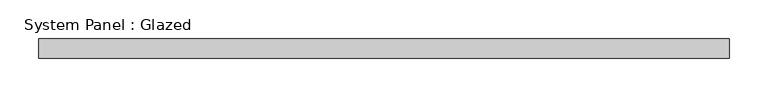
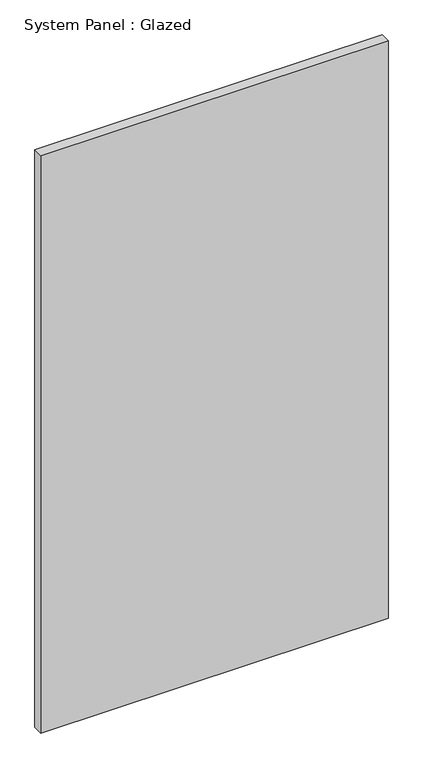
"""IFC4 building model written with IfcOpenShell, lengths in millimetres: plate geometry, System Panel : Glazed."""

from ifc_helpers import new_model, si_unit, origin, origin_with_axes, place, context, project, spatial, polyline, outline, extrude, source, transform, mapped, element, save


def system_panel_glazed_d1fbebc5(model_context):
    return source(origin(), model_context, "Body", "SweptSolid", [
        extrude(outline(polyline([(447.675, 19.05), (-447.675, 19.05), (-447.675, 44.45), (447.675, 44.45), (447.675, 19.05)])), origin_with_axes(), (0.0, 0.0, 1.0), 1573.4017583),
    ])


if __name__ == "__main__":
    model = new_model("IFC4")
    model_context = context("Model", 3, world=origin())
    ifc_project = project(units=[si_unit("LENGTHUNIT", "METRE", prefix="MILLI")], contexts=[model_context])
    site = spatial("IfcSite", under=ifc_project)
    building = spatial("IfcBuilding", under=site)
    placement = place(None, origin())
    system_panel_glazed_shape = system_panel_glazed_d1fbebc5(model_context)
    element("IfcPlate", 1, ObjectType="System Panel : Glazed", at=placement, inside=building, context=model_context, shape_type="MappedRepresentation", body=[
        mapped(system_panel_glazed_shape, transform((0.0, 0.0, 0.0), x_axis=(1.0, 0.0, 0.0), y_axis=(0.0, 1.0, 0.0), z_axis=(0.0, 0.0, 1.0))),
    ])
    save(model, "model.ifc")

# Revit data of these elements
# Type "System Panel : Glazed"
#   Construction Type Id = "GSP4R"
#   Analytic Construction = "1/8 in Pilkington single glazing"
#   Visual Light Transmittance = 0.9
#   Solar Heat Gain Coefficient = 0.86
#   Heat Transfer Coefficient (U) = 1.18115 BTU/(h·ft²·°F)
#   Define Thermal Properties by = 1
# Element 1 (IfcPlate, "System Panel : Glazed")
#   Materials on its faces: "Glass"
# Materials
#   "Glass": class "Glass", colour RGB 0 128 192, transparency 0.75, Description = "Soda Lime Glass", Cost = 0
